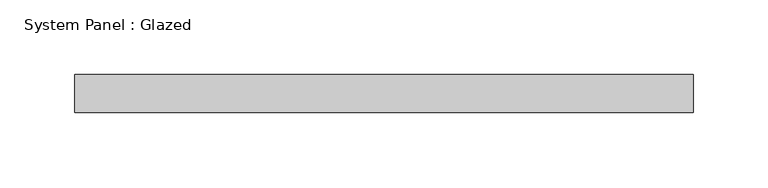
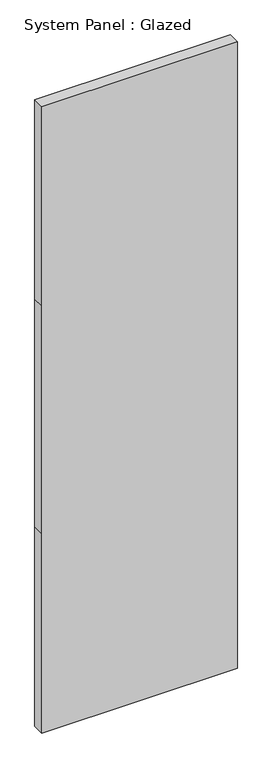
"""IFC4 building model written with IfcOpenShell, lengths in millimetres: plate geometry, System Panel : Glazed."""

from ifc_helpers import new_model, si_unit, frame, origin, place, context, project, spatial, polyline, outline, extrude, source, transform, mapped, element, save


def system_panel_glazed_26b8bff8(model_context):
    return source(origin(), model_context, "Body", "SweptSolid", [
        extrude(outline(polyline([(0.0, -206.375), (0.0, 206.375), (444.5, 206.375), (952.5, 206.375), (1397.0, 206.375), (1397.0, -206.375), (952.5, -206.375), (444.5, -206.375), (0.0, -206.375)])), frame((0.0, 19.05, 0.0), z_axis=(0.0, 1.0, 0.0), x_axis=(0.0, 0.0, 1.0)), (0.0, 0.0, 1.0), 25.4),
    ])


if __name__ == "__main__":
    model = new_model("IFC4")
    model_context = context("Model", 3, world=origin())
    ifc_project = project(units=[si_unit("LENGTHUNIT", "METRE", prefix="MILLI")], contexts=[model_context])
    site = spatial("IfcSite", under=ifc_project)
    building = spatial("IfcBuilding", under=site)
    placement = place(None, origin())
    system_panel_glazed_shape = system_panel_glazed_26b8bff8(model_context)
    element("IfcPlate", 1, ObjectType="System Panel : Glazed", at=placement, inside=building, context=model_context, shape_type="MappedRepresentation", body=[
        mapped(system_panel_glazed_shape, transform((0.0, 0.0, 0.0), x_axis=(1.0, 0.0, 0.0), y_axis=(0.0, 1.0, 0.0), z_axis=(0.0, 0.0, 1.0))),
    ])
    save(model, "model.ifc")

# Revit data of these elements
# Type "System Panel : Glazed"
#   Construction Type Id = "GSP4R"
#   Analytic Construction = "1/8 in Pilkington single glazing"
#   Visual Light Transmittance = 0.9
#   Solar Heat Gain Coefficient = 0.86
#   Heat Transfer Coefficient (U) = 1.18115 BTU/(h·ft²·°F)
#   Define Thermal Properties by = 1
# Element 1 (IfcPlate, "System Panel : Glazed")
#   Materials on its faces: "Glass"
# Materials
#   "Glass": class "Glass", colour RGB 0 128 192, transparency 0.75, Description = "Soda Lime Glass", Cost = 0
